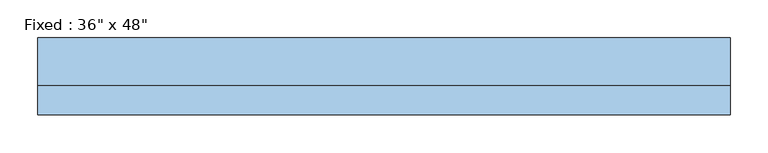
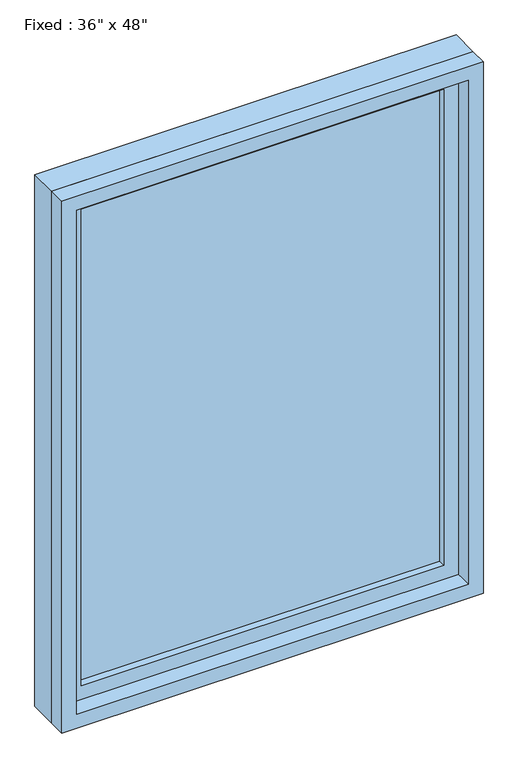
"""IFC4 building model written with IfcOpenShell, lengths in millimetres: window geometry."""

from ifc_helpers import new_model, si_unit, frame, origin, place, context, project, spatial, polyline, outline, extrude, source, transform, mapped, element, save


def window_d45db805(model_context):
    return source(origin(), model_context, "Body", "SweptSolid", [
        extrude(outline(polyline([(355.6, 3.175), (-431.8, 3.175), (-431.8, 15.875), (355.6, 15.875), (355.6, 3.175)])), frame((0.0, 0.0, 977.9), z_axis=(0.0, 0.0, 1.0), x_axis=(1.0, 0.0, 0.0)), (0.0, 0.0, 1.0), 1092.2),
        extrude(outline(polyline([(2114.55, -476.25), (933.45, -476.25), (933.45, 400.05), (2114.55, 400.05), (2114.55, -476.25)]), holes=[polyline([(2070.1, -431.8), (2070.1, 355.6), (977.9, 355.6), (977.9, -431.8), (2070.1, -431.8)])]), frame((0.0, -12.7, 0.0), z_axis=(0.0, 1.0, 0.0), x_axis=(0.0, 0.0, 1.0)), (0.0, 0.0, 1.0), 44.45),
        extrude(outline(polyline([(2133.6, -495.3), (914.4, -495.3), (914.4, 419.1), (2133.6, 419.1), (2133.6, -495.3)]), holes=[polyline([(2101.85, -463.55), (2101.85, 387.35), (946.15, 387.35), (946.15, -463.55), (2101.85, -463.55)])]), frame((0.0, -50.8, 0.0), z_axis=(0.0, 1.0, 0.0), x_axis=(0.0, 0.0, 1.0)), (0.0, 0.0, 1.0), 38.1),
        extrude(outline(polyline([(2133.6, 419.1), (2133.6, -495.3), (914.4, -495.3), (914.4, 419.1), (2133.6, 419.1)]), holes=[polyline([(2114.55, 400.05), (933.45, 400.05), (933.45, -476.25), (2114.55, -476.25), (2114.55, 400.05)])]), frame((0.0, -12.7, 0.0), z_axis=(0.0, 1.0, 0.0), x_axis=(0.0, 0.0, 1.0)), (0.0, 0.0, 1.0), 63.5),
    ])


if __name__ == "__main__":
    model = new_model("IFC4")
    model_context = context("Model", 3, world=origin())
    ifc_project = project(units=[si_unit("LENGTHUNIT", "METRE", prefix="MILLI")], contexts=[model_context])
    site = spatial("IfcSite", under=ifc_project)
    building = spatial("IfcBuilding", under=site)
    placement = place(None, origin())
    window_shape = window_d45db805(model_context)
    element("IfcWindow", 1, ObjectType="Fixed : 36\" x 48\"", at=placement, inside=building, context=model_context, shape_type="MappedRepresentation", body=[
        mapped(window_shape, transform((0.0, 0.0, 0.0), x_axis=(1.0, 0.0, 0.0), y_axis=(0.0, 1.0, 0.0), z_axis=(0.0, 0.0, 1.0))),
    ])
    save(model, "model.ifc")

# Revit data of these elements
# Type "Fixed : 36\" x 48\""
#   Type Mark = "1"
#   Construction Type Id = "GSP4R"
#   Assembly Code = "B2020100"
#   Analytic Construction = "1/8 in Pilkington single glazing"
#   Visual Light Transmittance = 0.9
#   Solar Heat Gain Coefficient = 0.78
#   Heat Transfer Coefficient (U) = 0.6496 BTU/(h·ft²·°F)
#   Height = 4' - 0"
#   Default Sill Height = 3' - 0"
#   Width = 3' - 0"
#   Window Inset = 0' - 0 3/4"
#   Define Thermal Properties by = 1
#   Glass Pane Material = Glass
#   Sash Material = Sash
#   Wall Closure = (empty or 0)
# Element 1 (IfcWindow, "Fixed : 36\" x 48\"")
#   Materials on its faces: "Sash", "Glass"
# Materials
#   "Glass": class "Glass", colour RGB 0 128 192, transparency 0.75, Description = "Soda Lime Glass", Cost = 0
#   "Sash": class "Wood", colour RGB 224 178 126, transparency 0
